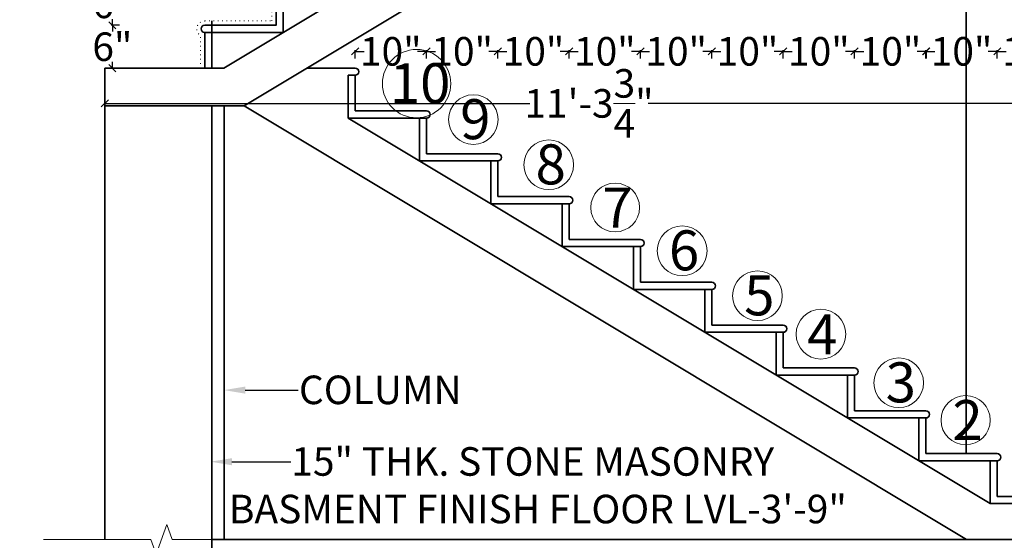
# Model space of a CAD drawing. Units: inches. Extents: x -60 to 284, y -245 to 257.
# Tile 3 of 10: x 55 to 193, y -159 to -86. Entities that reach past the tile are written whole.
import ezdxf
from ezdxf import colors
from ezdxf.entities.mleader import LeaderData, LeaderLine
from ezdxf.math import Vec2, Vec3

# ---------------------------------------------------------------- set-up
doc = ezdxf.new("R2010")
doc.units = ezdxf.units.IN
doc.header["$LTSCALE"] = 0.8
doc.header["$MEASUREMENT"] = 0
doc.linetypes.add('DOT', pattern=[6.35, 0, -6.35])
for name, color, linetype, lineweight in [('A-ANNO-DIMS', 2, 'Continuous', 18), ('A-ANNO-SYMB', 3, 'Continuous', 18), ('A-ANNO-TEXT', 3, 'Continuous', 18), ('A-SECT', 7, 'Continuous', 35), ('A-SECT-OVHD', 8, 'DOT', 18)]:
    doc.layers.add(name, color=color, linetype=linetype, lineweight=lineweight)
doc.styles.get("Standard").update_dxf_attribs({"font": 'arial.ttf'})
doc.dimstyles.get("Standard").update_dxf_attribs({"dimtxt": 4, "dimasz": 1, "dimexe": 0.18, "dimexo": 0.0625, "dimgap": 0.09, "dimtad": 0, "dimtih": 1, "dimtoh": 1, "dimzin": 0, "dimdsep": 46, "dimlunit": 4, "dimtxsty": 'Standard', "dimblk": 'OBLIQUE', "dimcen": 0.09, "dimadec": 0, "dimazin": 0, "dimtfac": 1, "dimtofl": 0, "dimtmove": 0, "dimatfit": 3, "dimfxl": 1, "dimfxlon": 1, "dimtolj": 1, "dimtzin": 0, "dimarcsym": 0})

# ---------------------------------------------------------------- blocks, each defined once
blk = doc.blocks.new('_Oblique')
at = {"color": 0, "linetype": 'ByBlock', "lineweight": -2}
blk.add_line((-0.5, -0.5), (0.5, 0.5), dxfattribs=at)
blk = doc.blocks.new('*D41')
at = {"layer": 'A-ANNO-DIMS', "color": 0, "lineweight": -2, "ltscale": 0.8, "transparency": 16777216}
for p, q in [((192.1, -91.86), (192.1, -90.68)), ((192.1, -90.86), (193.35, -90.86)), ((202.1, -90.86), (200.85, -90.86)), ((202.1, -91.86), (202.1, -90.68))]:
    blk.add_line(p, q, dxfattribs=at)
at = {"layer": 'Defpoints', "color": 0, "ltscale": 0.8, "transparency": 16777216}
for p in [(192.1, -90.86), (192.1, -168.75), (202.1, -168.75)]:
    blk.add_point(p, dxfattribs=at)
at = {"layer": 'A-ANNO-DIMS', "color": 0, "lineweight": -2, "ltscale": 0.8, "transparency": 16777216, "rotation": 180}
blk.add_blockref('_Oblique', (192.1, -90.86), dxfattribs=at)
at = {"layer": 'A-ANNO-DIMS', "color": 0, "lineweight": -2, "ltscale": 0.8, "transparency": 16777216}
blk.add_blockref('_Oblique', (202.1, -90.86), dxfattribs=at)
at = {"layer": 'A-ANNO-DIMS', "color": 0, "ltscale": 0.8, "transparency": 16777216, "insert": (197.1, -90.86), "char_height": 4, "attachment_point": 5}
blk.add_mtext('\\A1;10"', dxfattribs=at)
blk = doc.blocks.new('*D42')
at = {"layer": 'A-ANNO-DIMS', "color": 0, "lineweight": -2, "ltscale": 0.8, "transparency": 16777216}
for p, q in [((182.1, -91.86), (182.1, -90.68)), ((182.1, -90.86), (183.35, -90.86)), ((192.1, -90.86), (190.85, -90.86)), ((192.1, -91.86), (192.1, -90.68))]:
    blk.add_line(p, q, dxfattribs=at)
at = {"layer": 'Defpoints', "color": 0, "ltscale": 0.8, "transparency": 16777216}
for p in [(182.1, -90.86), (182.1, -162.75), (192.1, -162.75)]:
    blk.add_point(p, dxfattribs=at)
at = {"layer": 'A-ANNO-DIMS', "color": 0, "lineweight": -2, "ltscale": 0.8, "transparency": 16777216, "rotation": 180}
blk.add_blockref('_Oblique', (182.1, -90.86), dxfattribs=at)
at = {"layer": 'A-ANNO-DIMS', "color": 0, "lineweight": -2, "ltscale": 0.8, "transparency": 16777216}
blk.add_blockref('_Oblique', (192.1, -90.86), dxfattribs=at)
at = {"layer": 'A-ANNO-DIMS', "color": 0, "ltscale": 0.8, "transparency": 16777216, "insert": (187.1, -90.86), "char_height": 4, "attachment_point": 5}
blk.add_mtext('\\A1;10"', dxfattribs=at)
blk = doc.blocks.new('*D43')
at = {"layer": 'A-ANNO-DIMS', "color": 0, "lineweight": -2, "ltscale": 0.8, "transparency": 16777216}
for p, q in [((172.1, -91.86), (172.1, -90.68)), ((172.1, -90.86), (173.38, -90.86)), ((182.17, -90.86), (180.89, -90.86)), ((182.17, -91.86), (182.17, -90.68))]:
    blk.add_line(p, q, dxfattribs=at)
at = {"layer": 'Defpoints', "color": 0, "ltscale": 0.8, "transparency": 16777216}
for p in [(172.1, -90.86), (172.1, -156.75), (182.17, -156.76)]:
    blk.add_point(p, dxfattribs=at)
at = {"layer": 'A-ANNO-DIMS', "color": 0, "lineweight": -2, "ltscale": 0.8, "transparency": 16777216, "rotation": 180}
blk.add_blockref('_Oblique', (172.1, -90.86), dxfattribs=at)
at = {"layer": 'A-ANNO-DIMS', "color": 0, "lineweight": -2, "ltscale": 0.8, "transparency": 16777216}
blk.add_blockref('_Oblique', (182.17, -90.86), dxfattribs=at)
at = {"layer": 'A-ANNO-DIMS', "color": 0, "ltscale": 0.8, "transparency": 16777216, "insert": (177.14, -90.86), "char_height": 4, "attachment_point": 5}
blk.add_mtext('\\A1;10"', dxfattribs=at)
blk = doc.blocks.new('*D44')
at = {"layer": 'A-ANNO-DIMS', "color": 0, "lineweight": -2, "ltscale": 0.8, "transparency": 16777216}
for p, q in [((162.1, -91.86), (162.1, -90.68)), ((162.1, -90.86), (163.35, -90.86)), ((172.1, -90.86), (170.85, -90.86)), ((172.1, -91.86), (172.1, -90.68))]:
    blk.add_line(p, q, dxfattribs=at)
at = {"layer": 'Defpoints', "color": 0, "ltscale": 0.8, "transparency": 16777216}
for p in [(162.1, -90.86), (162.1, -150.75), (172.1, -150.75)]:
    blk.add_point(p, dxfattribs=at)
at = {"layer": 'A-ANNO-DIMS', "color": 0, "lineweight": -2, "ltscale": 0.8, "transparency": 16777216, "rotation": 180}
blk.add_blockref('_Oblique', (162.1, -90.86), dxfattribs=at)
at = {"layer": 'A-ANNO-DIMS', "color": 0, "lineweight": -2, "ltscale": 0.8, "transparency": 16777216}
blk.add_blockref('_Oblique', (172.1, -90.86), dxfattribs=at)
at = {"layer": 'A-ANNO-DIMS', "color": 0, "ltscale": 0.8, "transparency": 16777216, "insert": (167.1, -90.86), "char_height": 4, "attachment_point": 5}
blk.add_mtext('\\A1;10"', dxfattribs=at)
blk = doc.blocks.new('*D45')
at = {"layer": 'A-ANNO-DIMS', "color": 0, "lineweight": -2, "ltscale": 0.8, "transparency": 16777216}
for p, q in [((152.1, -91.86), (152.1, -90.68)), ((152.1, -90.86), (153.35, -90.86)), ((162.1, -90.86), (160.85, -90.86)), ((162.1, -91.86), (162.1, -90.68))]:
    blk.add_line(p, q, dxfattribs=at)
at = {"layer": 'Defpoints', "color": 0, "ltscale": 0.8, "transparency": 16777216}
for p in [(152.1, -90.86), (152.1, -144.75), (162.1, -144.75)]:
    blk.add_point(p, dxfattribs=at)
at = {"layer": 'A-ANNO-DIMS', "color": 0, "lineweight": -2, "ltscale": 0.8, "transparency": 16777216, "rotation": 180}
blk.add_blockref('_Oblique', (152.1, -90.86), dxfattribs=at)
at = {"layer": 'A-ANNO-DIMS', "color": 0, "lineweight": -2, "ltscale": 0.8, "transparency": 16777216}
blk.add_blockref('_Oblique', (162.1, -90.86), dxfattribs=at)
at = {"layer": 'A-ANNO-DIMS', "color": 0, "ltscale": 0.8, "transparency": 16777216, "insert": (157.1, -90.86), "char_height": 4, "attachment_point": 5}
blk.add_mtext('\\A1;10"', dxfattribs=at)
blk = doc.blocks.new('*D46')
at = {"layer": 'A-ANNO-DIMS', "color": 0, "lineweight": -2, "ltscale": 0.8, "transparency": 16777216}
for p, q in [((142.1, -91.86), (142.1, -90.68)), ((142.1, -90.86), (143.35, -90.86)), ((152.1, -90.86), (150.85, -90.86)), ((152.1, -91.86), (152.1, -90.68))]:
    blk.add_line(p, q, dxfattribs=at)
at = {"layer": 'Defpoints', "color": 0, "ltscale": 0.8, "transparency": 16777216}
for p in [(142.1, -90.86), (142.1, -138.75), (152.1, -138.75)]:
    blk.add_point(p, dxfattribs=at)
at = {"layer": 'A-ANNO-DIMS', "color": 0, "lineweight": -2, "ltscale": 0.8, "transparency": 16777216, "rotation": 180}
blk.add_blockref('_Oblique', (142.1, -90.86), dxfattribs=at)
at = {"layer": 'A-ANNO-DIMS', "color": 0, "lineweight": -2, "ltscale": 0.8, "transparency": 16777216}
blk.add_blockref('_Oblique', (152.1, -90.86), dxfattribs=at)
at = {"layer": 'A-ANNO-DIMS', "color": 0, "ltscale": 0.8, "transparency": 16777216, "insert": (147.1, -90.86), "char_height": 4, "attachment_point": 5}
blk.add_mtext('\\A1;10"', dxfattribs=at)
blk = doc.blocks.new('*D47')
at = {"layer": 'A-ANNO-DIMS', "color": 0, "lineweight": -2, "ltscale": 0.8, "transparency": 16777216}
for p, q in [((122.1, -91.86), (122.1, -90.68)), ((122.1, -90.86), (123.35, -90.86)), ((132.1, -90.86), (130.85, -90.86)), ((132.1, -91.86), (132.1, -90.68))]:
    blk.add_line(p, q, dxfattribs=at)
at = {"layer": 'Defpoints', "color": 0, "ltscale": 0.8, "transparency": 16777216}
for p in [(122.1, -90.86), (122.1, -126.75), (132.1, -126.75)]:
    blk.add_point(p, dxfattribs=at)
at = {"layer": 'A-ANNO-DIMS', "color": 0, "lineweight": -2, "ltscale": 0.8, "transparency": 16777216, "rotation": 180}
blk.add_blockref('_Oblique', (122.1, -90.86), dxfattribs=at)
at = {"layer": 'A-ANNO-DIMS', "color": 0, "lineweight": -2, "ltscale": 0.8, "transparency": 16777216}
blk.add_blockref('_Oblique', (132.1, -90.86), dxfattribs=at)
at = {"layer": 'A-ANNO-DIMS', "color": 0, "ltscale": 0.8, "transparency": 16777216, "insert": (127.1, -90.86), "char_height": 4, "attachment_point": 5}
blk.add_mtext('\\A1;10"', dxfattribs=at)
blk = doc.blocks.new('*D48')
at = {"layer": 'A-ANNO-DIMS', "color": 0, "lineweight": -2, "ltscale": 0.8, "transparency": 16777216}
for p, q in [((132.1, -91.86), (132.1, -90.68)), ((132.1, -90.86), (133.35, -90.86)), ((142.1, -90.86), (140.85, -90.86)), ((142.1, -91.86), (142.1, -90.68))]:
    blk.add_line(p, q, dxfattribs=at)
at = {"layer": 'Defpoints', "color": 0, "ltscale": 0.8, "transparency": 16777216}
for p in [(132.1, -90.86), (132.1, -132.75), (142.1, -132.75)]:
    blk.add_point(p, dxfattribs=at)
at = {"layer": 'A-ANNO-DIMS', "color": 0, "lineweight": -2, "ltscale": 0.8, "transparency": 16777216, "rotation": 180}
blk.add_blockref('_Oblique', (132.1, -90.86), dxfattribs=at)
at = {"layer": 'A-ANNO-DIMS', "color": 0, "lineweight": -2, "ltscale": 0.8, "transparency": 16777216}
blk.add_blockref('_Oblique', (142.1, -90.86), dxfattribs=at)
at = {"layer": 'A-ANNO-DIMS', "color": 0, "ltscale": 0.8, "transparency": 16777216, "insert": (137.1, -90.86), "char_height": 4, "attachment_point": 5}
blk.add_mtext('\\A1;10"', dxfattribs=at)
blk = doc.blocks.new('*D49')
at = {"layer": 'A-ANNO-DIMS', "color": 0, "lineweight": -2, "ltscale": 0.8, "transparency": 16777216}
for p, q in [((102.1, -91.86), (102.1, -90.68)), ((102.1, -90.86), (103.35, -90.86)), ((112.1, -90.86), (110.85, -90.86)), ((112.1, -91.86), (112.1, -90.68))]:
    blk.add_line(p, q, dxfattribs=at)
at = {"layer": 'Defpoints', "color": 0, "ltscale": 0.8, "transparency": 16777216}
for p in [(102.1, -90.86), (102.1, -99.21), (112.1, -99.21)]:
    blk.add_point(p, dxfattribs=at)
at = {"layer": 'A-ANNO-DIMS', "color": 0, "lineweight": -2, "ltscale": 0.8, "transparency": 16777216, "rotation": 180}
blk.add_blockref('_Oblique', (102.1, -90.86), dxfattribs=at)
at = {"layer": 'A-ANNO-DIMS', "color": 0, "lineweight": -2, "ltscale": 0.8, "transparency": 16777216}
blk.add_blockref('_Oblique', (112.1, -90.86), dxfattribs=at)
at = {"layer": 'A-ANNO-DIMS', "color": 0, "ltscale": 0.8, "transparency": 16777216, "insert": (107.1, -90.86), "char_height": 4, "attachment_point": 5}
blk.add_mtext('\\A1;10"', dxfattribs=at)
blk = doc.blocks.new('*D50')
at = {"layer": 'A-ANNO-DIMS', "color": 0, "lineweight": -2, "ltscale": 0.8, "transparency": 16777216}
for p, q in [((112.1, -91.86), (112.1, -90.68)), ((112.1, -90.86), (113.35, -90.86)), ((122.1, -90.86), (120.85, -90.86)), ((122.1, -91.86), (122.1, -90.68))]:
    blk.add_line(p, q, dxfattribs=at)
at = {"layer": 'Defpoints', "color": 0, "ltscale": 0.8, "transparency": 16777216}
for p in [(112.1, -90.86), (112.1, -105.21), (122.1, -105.21)]:
    blk.add_point(p, dxfattribs=at)
at = {"layer": 'A-ANNO-DIMS', "color": 0, "lineweight": -2, "ltscale": 0.8, "transparency": 16777216, "rotation": 180}
blk.add_blockref('_Oblique', (112.1, -90.86), dxfattribs=at)
at = {"layer": 'A-ANNO-DIMS', "color": 0, "lineweight": -2, "ltscale": 0.8, "transparency": 16777216}
blk.add_blockref('_Oblique', (122.1, -90.86), dxfattribs=at)
at = {"layer": 'A-ANNO-DIMS', "color": 0, "ltscale": 0.8, "transparency": 16777216, "insert": (117.1, -90.86), "char_height": 4, "attachment_point": 5}
blk.add_mtext('\\A1;10"', dxfattribs=at)
blk = doc.blocks.new('*D51')
at = {"layer": 'A-ANNO-DIMS', "color": 0, "lineweight": -2, "ltscale": 0.8, "transparency": 16777216}
for p, q in [((81.01, -30.69), (81.01, -29.51)), ((81.01, -29.69), (82.26, -29.69)), ((91.01, -29.69), (89.77, -29.69)), ((91.01, -30.69), (91.01, -29.51))]:
    blk.add_line(p, q, dxfattribs=at)
at = {"layer": 'Defpoints', "color": 0, "ltscale": 0.8, "transparency": 16777216}
for p in [(91.01, -29.69), (81.01, -87.21), (91.01, -87.21)]:
    blk.add_point(p, dxfattribs=at)
at = {"layer": 'A-ANNO-DIMS', "color": 0, "lineweight": -2, "ltscale": 0.8, "transparency": 16777216, "rotation": 180}
blk.add_blockref('_Oblique', (81.01, -29.69), dxfattribs=at)
at = {"layer": 'A-ANNO-DIMS', "color": 0, "lineweight": -2, "ltscale": 0.8, "transparency": 16777216}
blk.add_blockref('_Oblique', (91.01, -29.69), dxfattribs=at)
at = {"layer": 'A-ANNO-DIMS', "color": 0, "ltscale": 0.8, "transparency": 16777216, "insert": (86.01, -29.69), "char_height": 4, "attachment_point": 5}
blk.add_mtext('\\A1;10"', dxfattribs=at)
blk = doc.blocks.new('*D59')
at = {"layer": 'A-ANNO-DIMS', "color": 0, "lineweight": -2, "ltscale": 0.8, "transparency": 16777216}
for p, q in [((69.07, -87.21), (67.89, -87.21)), ((68.07, -87.21), (68.07, -88.08)), ((68.07, -93.21), (68.07, -92.34)), ((69.07, -93.21), (67.89, -93.21))]:
    blk.add_line(p, q, dxfattribs=at)
at = {"layer": 'Defpoints', "color": 0, "ltscale": 0.8, "transparency": 16777216}
for p in [(68.07, -87.21), (81.01, -87.21), (81.01, -93.21)]:
    blk.add_point(p, dxfattribs=at)
at = {"layer": 'A-ANNO-DIMS', "color": 0, "lineweight": -2, "ltscale": 0.8, "transparency": 16777216}
for p, rotation in [((68.07, -87.21), 90), ((68.07, -93.21), 270)]:
    blk.add_blockref('_Oblique', p, dxfattribs=dict(at, rotation=rotation))
at = {"layer": 'A-ANNO-DIMS', "color": 0, "ltscale": 0.8, "transparency": 16777216, "insert": (68.07, -90.21), "char_height": 4, "attachment_point": 5}
blk.add_mtext('\\A1;6"', dxfattribs=at)
blk = doc.blocks.new('*D60')
at = {"layer": 'A-ANNO-DIMS', "color": 0, "lineweight": -2, "ltscale": 0.8, "transparency": 16777216}
for p, q in [((69.07, -81.21), (67.89, -81.21)), ((68.07, -81.21), (68.07, -82.08)), ((68.07, -87.21), (68.07, -86.34)), ((69.07, -87.21), (67.89, -87.21))]:
    blk.add_line(p, q, dxfattribs=at)
at = {"layer": 'Defpoints', "color": 0, "ltscale": 0.8, "transparency": 16777216}
for p in [(68.07, -81.21), (91.01, -81.21), (91.01, -87.21)]:
    blk.add_point(p, dxfattribs=at)
at = {"layer": 'A-ANNO-DIMS', "color": 0, "lineweight": -2, "ltscale": 0.8, "transparency": 16777216}
for p, rotation in [((68.07, -81.21), 90), ((68.07, -87.21), 270)]:
    blk.add_blockref('_Oblique', p, dxfattribs=dict(at, rotation=rotation))
at = {"layer": 'A-ANNO-DIMS', "color": 0, "ltscale": 0.8, "transparency": 16777216, "insert": (68.07, -84.21), "char_height": 4, "attachment_point": 5}
blk.add_mtext('\\A1;6"', dxfattribs=at)
blk = doc.blocks.new('*D68')
at = {"layer": 'A-ANNO-DIMS', "color": 0, "lineweight": -2, "ltscale": 0.8, "transparency": 16777216}
for p, q in [((67.01, -97.15), (67.01, -98.33)), ((202.74, -97.15), (202.74, -98.33)), ((67.01, -98.15), (126.59, -98.15)), ((202.74, -98.15), (143.17, -98.15))]:
    blk.add_line(p, q, dxfattribs=at)
at = {"layer": 'Defpoints', "color": 0, "ltscale": 0.8, "transparency": 16777216}
for p in [(67.01, -93.21), (202.74, -93.21), (202.74, -98.15)]:
    blk.add_point(p, dxfattribs=at)
at = {"layer": 'A-ANNO-DIMS', "color": 0, "lineweight": -2, "ltscale": 0.8, "transparency": 16777216, "rotation": 180}
blk.add_blockref('_Oblique', (67.01, -98.15), dxfattribs=at)
at = {"layer": 'A-ANNO-DIMS', "color": 0, "lineweight": -2, "ltscale": 0.8, "transparency": 16777216}
blk.add_blockref('_Oblique', (202.74, -98.15), dxfattribs=at)
at = {"layer": 'A-ANNO-DIMS', "color": 0, "ltscale": 0.8, "transparency": 16777216, "insert": (134.88, -98.15), "char_height": 4, "attachment_point": 5}
blk.add_mtext('\\A1;11\'-3{\\H1x;\\S3/4;}"', dxfattribs=at)
blk = doc.blocks.new('*D72')
at = {"layer": 'A-ANNO-DIMS', "color": 0, "lineweight": -2, "ltscale": 0.8, "transparency": 16777216}
for p, q in [((67.01, -20.01), (67.01, -18.83)), ((67.01, -19.01), (68.51, -19.01)), ((68.51, -20.01), (68.51, -18.83)), ((68.51, -19.01), (69.51, -19.01))]:
    blk.add_line(p, q, dxfattribs=at)
at = {"layer": 'Defpoints', "color": 0, "ltscale": 0.8, "transparency": 16777216}
for p in [(68.51, -19.01), (67.01, -93.21), (68.51, -93.21)]:
    blk.add_point(p, dxfattribs=at)
at = {"layer": 'A-ANNO-DIMS', "color": 0, "lineweight": -2, "ltscale": 0.8, "transparency": 16777216, "rotation": 180}
blk.add_blockref('_Oblique', (67.01, -19.01), dxfattribs=at)
at = {"layer": 'A-ANNO-DIMS', "color": 0, "lineweight": -2, "ltscale": 0.8, "transparency": 16777216}
blk.add_blockref('_Oblique', (68.51, -19.01), dxfattribs=at)
at = {"layer": 'A-ANNO-DIMS', "color": 0, "ltscale": 0.8, "transparency": 16777216, "insert": (73.17, -19.01), "char_height": 4, "attachment_point": 5}
blk.add_mtext('\\A1;1{\\H1x;\\S1/2;}"', dxfattribs=at)
blk = doc.blocks.new('*D73')
at = {"layer": 'A-ANNO-DIMS', "color": 0, "lineweight": -2, "ltscale": 0.8, "transparency": 16777216}
for p, q in [((70.41, -31.19), (70.41, -30.01)), ((70.41, -30.19), (71.66, -30.19)), ((80.41, -30.19), (79.17, -30.19)), ((80.41, -31.19), (80.41, -30.01))]:
    blk.add_line(p, q, dxfattribs=at)
at = {"layer": 'Defpoints', "color": 0, "ltscale": 0.8, "transparency": 16777216}
for p in [(80.41, -30.19), (70.41, -93.21), (80.41, -93.21)]:
    blk.add_point(p, dxfattribs=at)
at = {"layer": 'A-ANNO-DIMS', "color": 0, "lineweight": -2, "ltscale": 0.8, "transparency": 16777216, "rotation": 180}
blk.add_blockref('_Oblique', (70.41, -30.19), dxfattribs=at)
at = {"layer": 'A-ANNO-DIMS', "color": 0, "lineweight": -2, "ltscale": 0.8, "transparency": 16777216}
blk.add_blockref('_Oblique', (80.41, -30.19), dxfattribs=at)
at = {"layer": 'A-ANNO-DIMS', "color": 0, "ltscale": 0.8, "transparency": 16777216, "insert": (75.41, -30.19), "char_height": 4, "attachment_point": 5}
blk.add_mtext('\\A1;10"', dxfattribs=at)
blk = doc.blocks.new('*D105')
at = {"layer": 'A-ANNO-DIMS', "color": 0, "lineweight": -2, "ltscale": 0.8, "transparency": 16777216}
for p, q in [((67.01, -241.38), (67.01, -242.56)), ((244.9, -241.38), (244.9, -242.56)), ((67.01, -242.38), (149.3, -242.38)), ((244.9, -242.38), (162.61, -242.38))]:
    blk.add_line(p, q, dxfattribs=at)
at = {"layer": 'Defpoints', "color": 0, "ltscale": 0.8, "transparency": 16777216}
for p in [(67.01, -159.21), (244.9, -171.21), (244.9, -242.38)]:
    blk.add_point(p, dxfattribs=at)
at = {"layer": 'A-ANNO-DIMS', "color": 0, "lineweight": -2, "ltscale": 0.8, "transparency": 16777216, "rotation": 180}
blk.add_blockref('_Oblique', (67.01, -242.38), dxfattribs=at)
at = {"layer": 'A-ANNO-DIMS', "color": 0, "lineweight": -2, "ltscale": 0.8, "transparency": 16777216}
blk.add_blockref('_Oblique', (244.9, -242.38), dxfattribs=at)
at = {"layer": 'A-ANNO-DIMS', "color": 0, "ltscale": 0.8, "transparency": 16777216, "insert": (155.96, -242.38), "char_height": 4, "attachment_point": 5}
blk.add_mtext('\\A1;177.9', dxfattribs=at)
blk = doc.blocks.new('*D106')
at = {"layer": 'A-ANNO-DIMS', "color": 0, "lineweight": -2, "ltscale": 0.8, "transparency": 16777216}
for p, q in [((-50.85, -93.21), (-52.03, -93.21)), ((-51.85, -93.21), (-51.85, -93.71)), ((-51.85, -98.48), (-51.85, -97.98)), ((-50.85, -98.48), (-52.03, -98.48))]:
    blk.add_line(p, q, dxfattribs=at)
at = {"layer": 'Defpoints', "color": 0, "ltscale": 0.8, "transparency": 16777216}
for p in [(67.01, -93.21), (-51.85, -98.48), (67.01, -98.48)]:
    blk.add_point(p, dxfattribs=at)
at = {"layer": 'A-ANNO-DIMS', "color": 0, "lineweight": -2, "ltscale": 0.8, "transparency": 16777216}
for p, rotation in [((-51.85, -93.21), 90), ((-51.85, -98.48), 270)]:
    blk.add_blockref('_Oblique', p, dxfattribs=dict(at, rotation=rotation))
at = {"layer": 'A-ANNO-DIMS', "color": 0, "ltscale": 0.8, "transparency": 16777216, "insert": (-51.85, -95.84), "char_height": 4, "attachment_point": 5}
blk.add_mtext('\\A1;5.271', dxfattribs=at)
blk = doc.blocks.new('*D113')
at = {"layer": 'A-ANNO-DIMS', "color": 0, "lineweight": -2, "ltscale": 0.8, "transparency": 16777216}
for p, q in [((67.01, 6.88), (67.01, 8.06)), ((67.01, 7.88), (67.14, 7.88)), ((83.68, 7.88), (83.55, 7.88)), ((83.68, 6.88), (83.68, 8.06))]:
    blk.add_line(p, q, dxfattribs=at)
at = {"layer": 'Defpoints', "color": 0, "ltscale": 0.8, "transparency": 16777216}
for p in [(83.68, 7.88), (67.01, -93.21), (83.68, -93.21)]:
    blk.add_point(p, dxfattribs=at)
at = {"layer": 'A-ANNO-DIMS', "color": 0, "lineweight": -2, "ltscale": 0.8, "transparency": 16777216, "rotation": 180}
blk.add_blockref('_Oblique', (67.01, 7.88), dxfattribs=at)
at = {"layer": 'A-ANNO-DIMS', "color": 0, "lineweight": -2, "ltscale": 0.8, "transparency": 16777216}
blk.add_blockref('_Oblique', (83.68, 7.88), dxfattribs=at)
at = {"layer": 'A-ANNO-DIMS', "color": 0, "ltscale": 0.8, "transparency": 16777216, "insert": (75.35, 7.88), "char_height": 4, "attachment_point": 5}
blk.add_mtext('\\A1;16.667', dxfattribs=at)

msp = doc.modelspace()

# ---------------------------------------------------------------- linework, layer by layer
at = {"layer": 'A-ANNO-SYMB', "ltscale": 0.8}
msp.add_lwpolyline([(82.1939, -159.2089), (76.4394, -159.2089), (75.6894, -157.1482), (74.1894, -161.2695), (73.4394, -159.2089), (58.3996, -159.2089)], dxfattribs=at)
for centre, radius in [((110.7045, -95.3856), 4.788), ((118.665, -100.4209), 3.4808), ((129.2336, -106.7477), 3.4829), ((138.5407, -112.7344), 3.4155), ((147.9321, -118.7911), 3.485), ((158.4901, -125.0848), 3.4796), ((167.3912, -130.4785), 3.4851), ((178.2939, -137.2866), 3.4782), ((187.6662, -142.5181), 3.4482)]:
    msp.add_circle(centre, radius, dxfattribs=at)
at = {"layer": 'A-SECT', "ltscale": 0.8}
for p, q in [((187.7426, -46.2089), (187.7426, -147.2089)), ((92.0139, -88.2089), (92.0139, -82.2089)), ((82.0139, -86.6089), (82.0139, -93.2089)), ((81.0139, -88.2089), (92.0139, -88.2089)), ((82.0139, -93.2089), (82.0139, -88.2089)), ((67.0139, -93.2089), (67.0139, -159.2089)), ((83.6806, -93.2089), (67.0139, -93.2089)), ((67.0139, -93.2089), (68.5139, -93.2089)), ((80.4139, -93.2089), (70.4139, -93.2089)), ((102.1002, -93.2089), (95.3425, -93.2089)), ((101.1002, -100.2089), (101.1002, -94.2089)), ((102.1002, -94.2089), (101.1002, -94.2089)), ((102.1002, -99.2089), (102.1002, -94.2089)), ((86.557, -98.4801), (67.0139, -98.4801)), ((82.0139, -98.4801), (82.0139, -159.2089)), ((83.7425, -98.4801), (83.7425, -159.2089)), ((112.1002, -99.2089), (102.1002, -99.2089)), ((112.1002, -100.2089), (101.1002, -100.2089)), ((111.1002, -106.2089), (111.1002, -100.2089)), ((112.1002, -105.2089), (112.1002, -100.2089)), ((122.1002, -106.2089), (111.1002, -106.2089)), ((122.1002, -105.2089), (112.1002, -105.2089)), ((121.1002, -112.2089), (121.1002, -106.2089)), ((122.1002, -111.2089), (122.1002, -106.2089)), ((132.1002, -111.2089), (122.1002, -111.2089)), ((132.1002, -112.2089), (121.1002, -112.2089)), ((131.1002, -118.2089), (131.1002, -112.2089)), ((132.1002, -117.2089), (132.1002, -112.2089)), ((142.1002, -117.2089), (132.1002, -117.2089)), ((142.1002, -118.2089), (131.1002, -118.2089)), ((141.1002, -124.2089), (141.1002, -118.2089)), ((142.1002, -123.2089), (142.1002, -118.2089)), ((152.1002, -123.2089), (142.1002, -123.2089)), ((152.1002, -124.2089), (141.1002, -124.2089)), ((151.1002, -130.2089), (151.1002, -124.2089)), ((152.1002, -129.2089), (152.1002, -124.2089)), ((162.1002, -129.2089), (152.1002, -129.2089)), ((162.1002, -130.2089), (151.1002, -130.2089)), ((161.1002, -136.2089), (161.1002, -130.2089)), ((162.1002, -135.2089), (162.1002, -130.2089)), ((172.1002, -135.2089), (162.1002, -135.2089)), ((172.1002, -136.2089), (161.1002, -136.2089)), ((171.1002, -142.2089), (171.1002, -136.2089)), ((172.1002, -141.2089), (172.1002, -136.2089)), ((182.1002, -141.2089), (172.1002, -141.2089)), ((182.1002, -142.2089), (171.1002, -142.2089)), ((181.1002, -148.2089), (181.1002, -142.2089)), ((182.1002, -147.2089), (182.1002, -142.2089)), ((192.1002, -147.2089), (182.1002, -147.2089)), ((192.1002, -148.2089), (181.1002, -148.2089)), ((191.1002, -154.2089), (191.1002, -148.2089)), ((192.1002, -153.2089), (192.1002, -148.2089)), ((202.1002, -154.2089), (191.1002, -154.2089)), ((202.1002, -153.2089), (192.1002, -153.2089)), ((244.8977, -159.2089), (82.0139, -159.2089)), ((82.0139, -159.2089), (82.0139, -171.2089)), ((187.7426, -159.1914), (187.7426, -159.2089))]:
    msp.add_line(p, q, dxfattribs=at)
for points in [[(162.0139, -46.2089), (83.6806, -93.2089)], [(173.6758, -46.2089), (86.557, -98.4801)], [(86.557, -98.4801), (187.7716, -159.2089)], [(101.1002, -100.2089), (191.1002, -154.2089)]]:
    msp.add_lwpolyline(points, dxfattribs=at)
msp.add_lwpolyline([(81.0139, -93.2089), (81.0139, -88.2089, -1), (81.0139, -87.2089), (91.0139, -87.2089), (91.0139, -82.2089, -1)], format="xyb", dxfattribs=at)
for centre in [(102.1002, -93.7089), (112.1002, -99.7089), (122.1002, -105.7089), (132.1002, -111.7089), (142.1002, -117.7089), (152.1002, -123.7089), (162.1002, -129.7089), (172.1002, -135.7089), (182.1002, -141.7089), (192.1002, -147.7089)]:
    msp.add_arc(centre, 0.5, 270, 90, dxfattribs=at)
at = {"layer": 'A-SECT-OVHD', "ltscale": 0.1}
msp.add_lwpolyline([(80.4139, -93.2089), (80.4139, -88.6308, -0.74635672), (81.0139, -86.6089), (90.4139, -86.6089), (90.4139, -82.6308, -0.74635672)], format="xyb", dxfattribs=at)

# ---------------------------------------------------------------- texts
at = {"layer": 'A-ANNO-TEXT', "ltscale": 0.8, "attachment_point": 1}
for s, width, gutter_width, insert, char_height in [('10', 28.020867, 2.8021, (106.9639, -92.5242), 5.60417), ('9', 28.020867, 2.8021, (116.8224, -97.5596), 5.6042), ('8', 28.020867, 2.8021, (127.3872, -103.8863), 5.6042), ('7', 28.020867, 2.8021, (136.7268, -109.9324), 5.6042), ('6', 28.020867, 2.8021, (146.0819, -115.9298), 5.6042), ('5', 28.020867, 2.8021, (156.6322, -122.235), 5.6042), ('4', 28.020867, 2.8021, (165.453, -127.6764), 5.6042), ('3', 28.020867, 2.8021, (176.459, -134.4233), 5.6042), ('2', 28.020867, 2.8021, (185.8102, -139.7045), 5.6042), ('BASMENT FINISH FLOOR LVL-3\'-9"', 97.551324, 1, (84.4, -152.966), 4)]:
    msp.add_mtext_dynamic_manual_height_columns(s, width=width, gutter_width=gutter_width, heights=[0], dxfattribs=dict(at, insert=insert, char_height=char_height))

# ---------------------------------------------------------------- dimensions: what is measured, and where the dimension line sits
at = {"layer": 'A-ANNO-DIMS', "ltscale": 0.8}
for base, p1, p2, override, picture, middle in [((83.6806, 7.877), (67.0139, -93.2089), (83.6806, -93.2089), {"dimdec": 3, "dimlfac": 1, "dimrnd": 0, "dimzin": 0, "dimdsep": 46, "dimlunit": 2}, '*D113', (75.3472, 7.877)), ((68.5139, -19.0057), (67.0139, -93.2089), (68.5139, -93.2089), {"dimclrd": 0, "dimclre": 0, "dimclrt": 0}, '*D72', (73.1728, -19.0057)), ((80.4139, -30.1873), (70.4139, -93.2089), (80.4139, -93.2089), {"dimclrd": 0, "dimclre": 0, "dimclrt": 0}, '*D73', (75.4139, -30.1873)), ((91.0139, -29.6873), (81.0139, -87.2089), (91.0139, -87.2089), {"dimclrd": 0, "dimclre": 0, "dimclrt": 0}, '*D51', (86.0139, -29.6873)), ((102.1002, -90.8616), (112.1002, -99.2089), (102.1002, -99.2089), {"dimclrd": 0, "dimclre": 0, "dimclrt": 0}, '*D49', (107.1002, -90.8616)), ((112.1002, -90.8616), (122.1002, -105.2089), (112.1002, -105.2089), {"dimclrd": 0, "dimclre": 0, "dimclrt": 0}, '*D50', (117.1002, -90.8616)), ((122.1002, -90.8616), (132.1002, -126.7549), (122.1002, -126.7549), {"dimclrd": 0, "dimclre": 0, "dimclrt": 0}, '*D47', (127.1002, -90.8616)), ((132.1002, -90.8616), (142.1002, -132.7549), (132.1002, -132.7549), {"dimclrd": 0, "dimclre": 0, "dimclrt": 0}, '*D48', (137.1002, -90.8616)), ((142.1002, -90.8616), (152.1002, -138.7549), (142.1002, -138.7549), {"dimclrd": 0, "dimclre": 0, "dimclrt": 0}, '*D46', (147.1002, -90.8616)), ((152.1002, -90.8616), (162.1002, -144.7549), (152.1002, -144.7549), {"dimclrd": 0, "dimclre": 0, "dimclrt": 0}, '*D45', (157.1002, -90.8616)), ((162.1002, -90.8616), (172.1002, -150.7549), (162.1002, -150.7549), {"dimclrd": 0, "dimclre": 0, "dimclrt": 0}, '*D44', (167.1002, -90.8616)), ((172.1002, -90.8616), (182.1747, -156.7605), (172.1002, -156.7549), {"dimclrd": 0, "dimclre": 0, "dimclrt": 0}, '*D43', (177.1374, -90.8616)), ((182.1002, -90.8616), (192.1002, -162.7549), (182.1002, -162.7549), {"dimclrd": 0, "dimclre": 0, "dimclrt": 0}, '*D42', (187.1002, -90.8616)), ((192.1002, -90.8616), (202.1002, -168.7549), (192.1002, -168.7549), {"dimclrd": 0, "dimclre": 0, "dimclrt": 0}, '*D41', (197.1002, -90.8616)), ((202.7426, -98.1513), (67.0139, -93.2089), (202.7426, -93.2089), {"dimclrd": 0, "dimclre": 0, "dimclrt": 0}, '*D68', (134.8782, -98.1513)), ((244.8977, -242.3835), (67.0139, -159.2089), (244.8977, -171.2089), {"dimdec": 1, "dimlfac": 1, "dimrnd": 0, "dimzin": 0, "dimdsep": 46, "dimlunit": 2}, '*D105', (155.9558, -242.3835))]:
    dim = msp.add_linear_dim(base=base, p1=p1, p2=p2, dimstyle='Standard', override=override, dxfattribs=at)
    dim.commit()
    dim.dimension.update_dxf_attribs({"geometry": picture, "text_midpoint": middle})
for base, p1, p2, override, picture, middle in [((68.0702, -81.2089), (91.0139, -87.2089), (91.0139, -81.2089), {"dimclrd": 0, "dimclre": 0, "dimclrt": 0}, '*D60', (68.0702, -84.2089)), ((68.0702, -87.2089), (81.0139, -93.2089), (81.0139, -87.2089), {"dimclrd": 0, "dimclre": 0, "dimclrt": 0}, '*D59', (68.0702, -90.2089)), ((-51.8489, -98.4801), (67.0139, -93.2089), (67.0139, -98.4801), {"dimdec": 3, "dimlfac": 1, "dimrnd": 0, "dimzin": 0, "dimdsep": 46, "dimlunit": 2}, '*D106', (-51.8489, -95.8445))]:
    dim = msp.add_linear_dim(base=base, p1=p1, p2=p2, angle=90, dimstyle='Standard', override=override, dxfattribs=at)
    dim.commit()
    dim.dimension.update_dxf_attribs({"geometry": picture, "text_midpoint": middle})

# ---------------------------------------------------------------- leaders
at = {"layer": 'A-ANNO-TEXT', "ltscale": 0.8}
ml = msp.add_multileader_mtext('Standard', dxfattribs=at)
ml.set_content('COLUMN', color=256)
ml.set_leader_properties()
ml.build(insert=Vec2(0, 0))
ml.multileader.update_dxf_attribs({"dogleg_length": 0.36, "arrow_head_size": 3})
ctx = ml.context
ctx.base_point, ctx.arrow_head_size, ctx.landing_gap_size, ctx.plane_origin = Vec3(94.1341, -138.3081), 3, 0.09, Vec3(83.6948, -138.3081)
notes = []
notes.append((ctx, [(0, (1, 1, 0), (93.7741, -138.3081), (1, 0), 0.36, [(0, [(83.6948, -138.3081)], 0, [])])]))
ctx.mtext.insert, ctx.mtext.flow_direction = Vec3(94.2241, -136.274), 5
ml = msp.add_multileader_mtext('Standard', dxfattribs=at)
ml.set_content('15" THK. STONE MASONRY', color=256)
ml.set_leader_properties()
ml.build(insert=Vec2(0, 0))
ml.multileader.update_dxf_attribs({"dogleg_length": 0.36, "arrow_head_size": 3})
ctx = ml.context
ctx.base_point, ctx.arrow_head_size, ctx.landing_gap_size, ctx.plane_origin = Vec3(93.0628, -148.337), 3, 0.09, Vec3(81.8179, -148.337)
notes.append((ctx, [(0, (1, 1, 0), (92.7028, -148.337), (1, 0), 0.36, [(0, [(81.8179, -148.337)], 0, [])])]))
ctx.mtext.insert, ctx.mtext.flow_direction = Vec3(93.1528, -146.3029), 5
for ctx, leaders in notes:
    for number, flags, end, landing, length, lines in leaders:
        leader = LeaderData()
        leader.index, (leader.has_last_leader_line, leader.has_dogleg_vector, leader.attachment_direction) = number, flags
        leader.last_leader_point, leader.dogleg_vector, leader.dogleg_length = Vec3(end), Vec3(landing), length
        for number, points, colour, breaks in lines:
            line = LeaderLine()
            line.index, line.vertices, line.color, line.breaks = number, Vec3.list(points), colors.encode_raw_color(colour), breaks
            leader.lines.append(line)
        ctx.leaders.append(leader)

doc.saveas('drawing.dxf')
